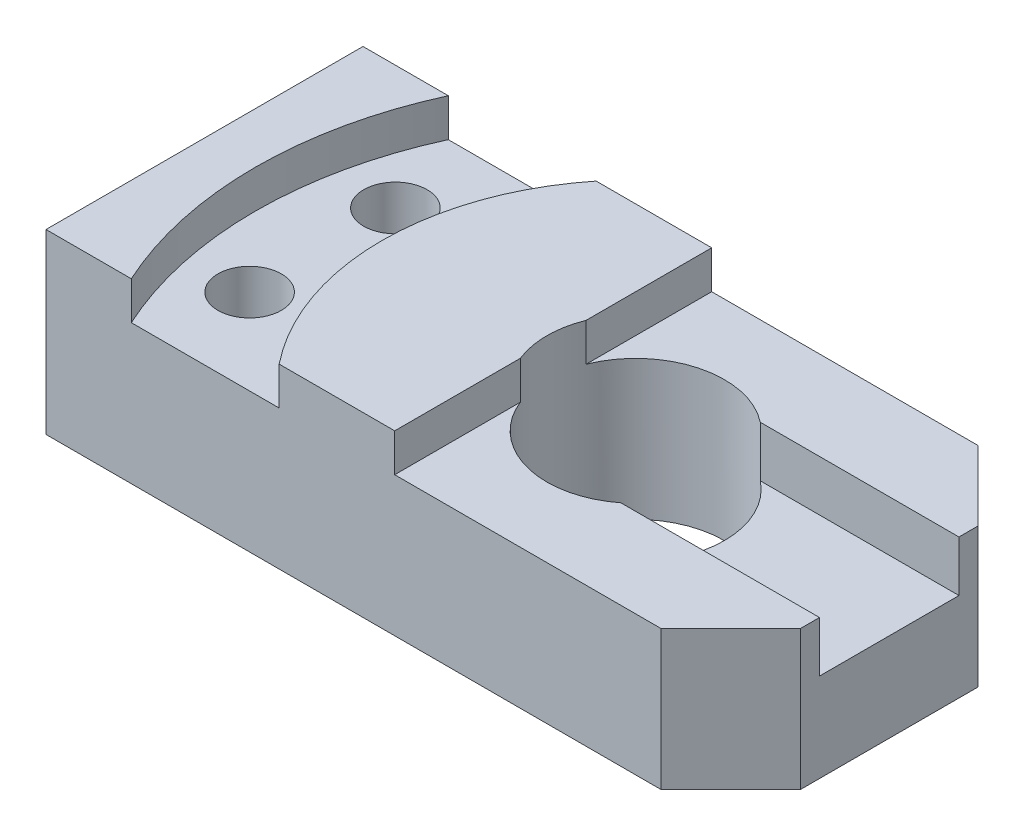
ISO-10303-21;
HEADER;
FILE_DESCRIPTION(('STEP AP214'),'2;1');
FILE_NAME('part.step','',(''),(''),'','','');
FILE_SCHEMA(('AUTOMOTIVE_DESIGN { 1 0 10303 214 1 1 1 1 }'));
ENDSEC;
DATA;
#1=APPLICATION_CONTEXT('core data for automotive mechanical design processes');
#2=APPLICATION_PROTOCOL_DEFINITION('international standard','automotive_design',2000,#1);
#3=PRODUCT_CONTEXT('',#1,'mechanical');
#4=PRODUCT('Part','Part','',(#3));
#5=PRODUCT_RELATED_PRODUCT_CATEGORY('part','',(#4));
#6=PRODUCT_DEFINITION_FORMATION('','',#4);
#7=PRODUCT_DEFINITION_CONTEXT('part definition',#1,'design');
#8=PRODUCT_DEFINITION('design','',#6,#7);
#9=PRODUCT_DEFINITION_SHAPE('','',#8);
#10=(LENGTH_UNIT() NAMED_UNIT(*) SI_UNIT(.MILLI.,.METRE.));
#11=(NAMED_UNIT(*) PLANE_ANGLE_UNIT() SI_UNIT($,.RADIAN.));
#12=(NAMED_UNIT(*) SI_UNIT($,.STERADIAN.) SOLID_ANGLE_UNIT());
#13=UNCERTAINTY_MEASURE_WITH_UNIT(LENGTH_MEASURE(1.E-05),#10,'distance_accuracy_value','');
#14=(GEOMETRIC_REPRESENTATION_CONTEXT(3) GLOBAL_UNCERTAINTY_ASSIGNED_CONTEXT((#13)) GLOBAL_UNIT_ASSIGNED_CONTEXT((#10,
#11,#12)) REPRESENTATION_CONTEXT('',''));
#15=CARTESIAN_POINT('',(0.,0.,0.));
#16=DIRECTION('',(0.,0.,1.));
#17=DIRECTION('',(1.,0.,0.));
#18=AXIS2_PLACEMENT_3D('',#15,#16,#17);
#19=CARTESIAN_POINT('',(0.,28.,0.));
#20=DIRECTION('',(0.,1.,0.));
#21=DIRECTION('',(0.,0.,1.));
#22=AXIS2_PLACEMENT_3D('',#19,#20,#21);
#23=PLANE('',#22);
#24=CARTESIAN_POINT('',(14.,28.,0.));
#25=DIRECTION('',(0.,-1.,0.));
#26=DIRECTION('',(0.,0.,1.));
#27=AXIS2_PLACEMENT_3D('',#24,#25,#26);
#28=CIRCLE('',#27,40.);
#29=CARTESIAN_POINT('',(-17.224989991992,28.,25.));
#30=VERTEX_POINT('',#29);
#31=CARTESIAN_POINT('',(-17.224989991992,28.,-25.));
#32=VERTEX_POINT('',#31);
#33=EDGE_CURVE('E176',#30,#32,#28,.T.);
#34=ORIENTED_EDGE('',*,*,#33,.F.);
#35=DIRECTION('',(1.,0.,0.));
#36=VECTOR('',#35,1.);
#37=CARTESIAN_POINT('',(-54.,28.,25.));
#38=LINE('',#37,#36);
#39=CARTESIAN_POINT('',(1.,28.,25.));
#40=VERTEX_POINT('',#39);
#41=EDGE_CURVE('E257',#30,#40,#38,.T.);
#42=ORIENTED_EDGE('',*,*,#41,.T.);
#43=DIRECTION('',(0.,0.,1.));
#44=VECTOR('',#43,1.);
#45=CARTESIAN_POINT('',(1.,28.,11.));
#46=LINE('',#45,#44);
#47=CARTESIAN_POINT('',(1.,28.,5.19615242270664));
#48=VERTEX_POINT('',#47);
#49=EDGE_CURVE('E231',#48,#40,#46,.T.);
#50=ORIENTED_EDGE('',*,*,#49,.F.);
#51=CARTESIAN_POINT('',(14.,28.,0.));
#52=DIRECTION('',(0.,1.,0.));
#53=DIRECTION('',(0.,0.,1.));
#54=AXIS2_PLACEMENT_3D('',#51,#52,#53);
#55=CIRCLE('',#54,14.);
#56=CARTESIAN_POINT('',(1.,28.,-5.19615242270664));
#57=VERTEX_POINT('',#56);
#58=EDGE_CURVE('E239',#57,#48,#55,.T.);
#59=ORIENTED_EDGE('',*,*,#58,.F.);
#60=CARTESIAN_POINT('',(1.,28.,-25.));
#61=VERTEX_POINT('',#60);
#62=EDGE_CURVE('E234',#61,#57,#46,.T.);
#63=ORIENTED_EDGE('',*,*,#62,.F.);
#64=DIRECTION('',(-1.,0.,0.));
#65=VECTOR('',#64,1.);
#66=CARTESIAN_POINT('',(54.,28.,-25.));
#67=LINE('',#66,#65);
#68=EDGE_CURVE('E252',#61,#32,#67,.T.);
#69=ORIENTED_EDGE('',*,*,#68,.T.);
#70=EDGE_LOOP('',(#34,#42,#50,#59,#63,#69));
#71=FACE_BOUND('',#70,.T.);
#72=ADVANCED_FACE('F43',(#71),#23,.T.);
#73=CARTESIAN_POINT('',(14.,22.,11.));
#74=DIRECTION('',(0.,-1.,0.));
#75=DIRECTION('',(0.,0.,-1.));
#76=AXIS2_PLACEMENT_3D('',#73,#74,#75);
#77=PLANE('',#76);
#78=DIRECTION('',(1.,0.,0.));
#79=VECTOR('',#78,1.);
#80=CARTESIAN_POINT('',(1.,22.,25.));
#81=LINE('',#80,#79);
#82=CARTESIAN_POINT('',(1.,22.,25.));
#83=VERTEX_POINT('',#82);
#84=CARTESIAN_POINT('',(43.,22.,25.));
#85=VERTEX_POINT('',#84);
#86=EDGE_CURVE('E236',#83,#85,#81,.T.);
#87=ORIENTED_EDGE('',*,*,#86,.T.);
#88=DIRECTION('',(-0.707106781186548,0.,0.707106781186547));
#89=VECTOR('',#88,1.);
#90=CARTESIAN_POINT('',(54.,22.,14.));
#91=LINE('',#90,#89);
#92=CARTESIAN_POINT('',(54.,22.,14.));
#93=VERTEX_POINT('',#92);
#94=EDGE_CURVE('E11',#85,#93,#91,.F.);
#95=ORIENTED_EDGE('',*,*,#94,.T.);
#96=DIRECTION('',(0.,0.,-1.));
#97=VECTOR('',#96,1.);
#98=CARTESIAN_POINT('',(54.,22.,11.));
#99=LINE('',#98,#97);
#100=CARTESIAN_POINT('',(54.,22.,11.));
#101=VERTEX_POINT('',#100);
#102=EDGE_CURVE('E247',#93,#101,#99,.T.);
#103=ORIENTED_EDGE('',*,*,#102,.T.);
#104=DIRECTION('',(1.,0.,0.));
#105=VECTOR('',#104,1.);
#106=CARTESIAN_POINT('',(14.,22.,11.));
#107=LINE('',#106,#105);
#108=CARTESIAN_POINT('',(22.6602540378444,22.,11.));
#109=VERTEX_POINT('',#108);
#110=EDGE_CURVE('E213',#109,#101,#107,.T.);
#111=ORIENTED_EDGE('',*,*,#110,.F.);
#112=CARTESIAN_POINT('',(14.,22.,0.));
#113=DIRECTION('',(0.,-1.,0.));
#114=DIRECTION('',(0.,0.,-1.));
#115=AXIS2_PLACEMENT_3D('',#112,#113,#114);
#116=CIRCLE('',#115,14.);
#117=CARTESIAN_POINT('',(1.,22.,5.19615242270664));
#118=VERTEX_POINT('',#117);
#119=EDGE_CURVE('E273',#109,#118,#116,.T.);
#120=ORIENTED_EDGE('',*,*,#119,.T.);
#121=DIRECTION('',(0.,0.,-1.));
#122=VECTOR('',#121,1.);
#123=CARTESIAN_POINT('',(1.,22.,25.));
#124=LINE('',#123,#122);
#125=EDGE_CURVE('E226',#83,#118,#124,.T.);
#126=ORIENTED_EDGE('',*,*,#125,.F.);
#127=EDGE_LOOP('',(#87,#95,#103,#111,#120,#126));
#128=FACE_BOUND('',#127,.T.);
#129=ADVANCED_FACE('F336',(#128),#77,.F.);
#130=CARTESIAN_POINT('',(14.,28.,0.));
#131=DIRECTION('',(0.,1.,0.));
#132=DIRECTION('',(0.,0.,1.));
#133=AXIS2_PLACEMENT_3D('',#130,#131,#132);
#134=CIRCLE('',#133,60.);
#135=CARTESIAN_POINT('',(-40.5435605731786,28.,-25.));
#136=VERTEX_POINT('',#135);
#137=CARTESIAN_POINT('',(-40.5435605731786,28.,25.));
#138=VERTEX_POINT('',#137);
#139=EDGE_CURVE('E186',#136,#138,#134,.T.);
#140=ORIENTED_EDGE('',*,*,#139,.F.);
#141=CARTESIAN_POINT('',(-54.,28.,-25.));
#142=VERTEX_POINT('',#141);
#143=EDGE_CURVE('E251',#136,#142,#67,.T.);
#144=ORIENTED_EDGE('',*,*,#143,.T.);
#145=DIRECTION('',(0.,0.,1.));
#146=VECTOR('',#145,1.);
#147=CARTESIAN_POINT('',(-54.,28.,-25.));
#148=LINE('',#147,#146);
#149=CARTESIAN_POINT('',(-54.,28.,25.));
#150=VERTEX_POINT('',#149);
#151=EDGE_CURVE('E254',#142,#150,#148,.T.);
#152=ORIENTED_EDGE('',*,*,#151,.T.);
#153=EDGE_CURVE('E260',#150,#138,#38,.T.);
#154=ORIENTED_EDGE('',*,*,#153,.T.);
#155=EDGE_LOOP('',(#140,#144,#152,#154));
#156=FACE_BOUND('',#155,.T.);
#157=ADVANCED_FACE('F342',(#156),#23,.T.);
#158=CARTESIAN_POINT('',(54.,28.,25.));
#159=DIRECTION('',(-1.,0.,0.));
#160=DIRECTION('',(0.,0.,1.));
#161=AXIS2_PLACEMENT_3D('',#158,#159,#160);
#162=PLANE('',#161);
#163=DIRECTION('',(0.,0.,-1.));
#164=VECTOR('',#163,1.);
#165=CARTESIAN_POINT('',(54.,0.,25.));
#166=LINE('',#165,#164);
#167=CARTESIAN_POINT('',(54.,0.,14.));
#168=VERTEX_POINT('',#167);
#169=CARTESIAN_POINT('',(54.,0.,-14.));
#170=VERTEX_POINT('',#169);
#171=EDGE_CURVE('E249',#168,#170,#166,.T.);
#172=ORIENTED_EDGE('',*,*,#171,.T.);
#173=DIRECTION('',(0.,1.,0.));
#174=VECTOR('',#173,1.);
#175=CARTESIAN_POINT('',(54.,28.,-14.));
#176=LINE('',#175,#174);
#177=CARTESIAN_POINT('',(54.,22.,-14.));
#178=VERTEX_POINT('',#177);
#179=EDGE_CURVE('E303',#170,#178,#176,.T.);
#180=ORIENTED_EDGE('',*,*,#179,.T.);
#181=CARTESIAN_POINT('',(54.,22.,-11.));
#182=VERTEX_POINT('',#181);
#183=EDGE_CURVE('E244',#182,#178,#99,.T.);
#184=ORIENTED_EDGE('',*,*,#183,.F.);
#185=DIRECTION('',(0.,1.,0.));
#186=VECTOR('',#185,1.);
#187=CARTESIAN_POINT('',(54.,22.,-11.));
#188=LINE('',#187,#186);
#189=CARTESIAN_POINT('',(54.,14.,-11.));
#190=VERTEX_POINT('',#189);
#191=EDGE_CURVE('E215',#190,#182,#188,.T.);
#192=ORIENTED_EDGE('',*,*,#191,.F.);
#193=DIRECTION('',(0.,0.,-1.));
#194=VECTOR('',#193,1.);
#195=CARTESIAN_POINT('',(54.,14.,11.));
#196=LINE('',#195,#194);
#197=CARTESIAN_POINT('',(54.,14.,11.));
#198=VERTEX_POINT('',#197);
#199=EDGE_CURVE('E209',#198,#190,#196,.T.);
#200=ORIENTED_EDGE('',*,*,#199,.F.);
#201=DIRECTION('',(0.,-1.,0.));
#202=VECTOR('',#201,1.);
#203=CARTESIAN_POINT('',(54.,22.,11.));
#204=LINE('',#203,#202);
#205=EDGE_CURVE('E204',#101,#198,#204,.T.);
#206=ORIENTED_EDGE('',*,*,#205,.F.);
#207=ORIENTED_EDGE('',*,*,#102,.F.);
#208=DIRECTION('',(0.,-1.,0.));
#209=VECTOR('',#208,1.);
#210=CARTESIAN_POINT('',(54.,28.,14.));
#211=LINE('',#210,#209);
#212=EDGE_CURVE('E297',#93,#168,#211,.T.);
#213=ORIENTED_EDGE('',*,*,#212,.T.);
#214=EDGE_LOOP('',(#172,#180,#184,#192,#200,#206,#207,#213));
#215=FACE_BOUND('',#214,.T.);
#216=ADVANCED_FACE('F352',(#215),#162,.F.);
#217=CARTESIAN_POINT('',(-54.,28.,-25.));
#218=DIRECTION('',(0.,0.,1.));
#219=DIRECTION('',(1.,0.,0.));
#220=AXIS2_PLACEMENT_3D('',#217,#218,#219);
#221=PLANE('',#220);
#222=DIRECTION('',(-1.,0.,0.));
#223=VECTOR('',#222,1.);
#224=CARTESIAN_POINT('',(-17.224989991992,22.,-25.));
#225=LINE('',#224,#223);
#226=CARTESIAN_POINT('',(-17.224989991992,22.,-25.));
#227=VERTEX_POINT('',#226);
#228=CARTESIAN_POINT('',(-40.5435605731786,22.,-25.));
#229=VERTEX_POINT('',#228);
#230=EDGE_CURVE('E184',#227,#229,#225,.T.);
#231=ORIENTED_EDGE('',*,*,#230,.F.);
#232=DIRECTION('',(0.,1.,0.));
#233=VECTOR('',#232,1.);
#234=CARTESIAN_POINT('',(-17.224989991992,22.,-25.));
#235=LINE('',#234,#233);
#236=EDGE_CURVE('E171',#227,#32,#235,.T.);
#237=ORIENTED_EDGE('',*,*,#236,.T.);
#238=ORIENTED_EDGE('',*,*,#68,.F.);
#239=DIRECTION('',(0.,1.,0.));
#240=VECTOR('',#239,1.);
#241=CARTESIAN_POINT('',(1.,28.,-25.));
#242=LINE('',#241,#240);
#243=CARTESIAN_POINT('',(1.,22.,-25.));
#244=VERTEX_POINT('',#243);
#245=EDGE_CURVE('E233',#244,#61,#242,.T.);
#246=ORIENTED_EDGE('',*,*,#245,.F.);
#247=DIRECTION('',(1.,0.,0.));
#248=VECTOR('',#247,1.);
#249=CARTESIAN_POINT('',(1.,22.,-25.));
#250=LINE('',#249,#248);
#251=CARTESIAN_POINT('',(43.,22.,-25.));
#252=VERTEX_POINT('',#251);
#253=EDGE_CURVE('E240',#244,#252,#250,.T.);
#254=ORIENTED_EDGE('',*,*,#253,.T.);
#255=DIRECTION('',(0.,-1.,0.));
#256=VECTOR('',#255,1.);
#257=CARTESIAN_POINT('',(43.,28.,-25.));
#258=LINE('',#257,#256);
#259=CARTESIAN_POINT('',(43.,0.,-25.));
#260=VERTEX_POINT('',#259);
#261=EDGE_CURVE('E291',#252,#260,#258,.T.);
#262=ORIENTED_EDGE('',*,*,#261,.T.);
#263=DIRECTION('',(-1.,0.,0.));
#264=VECTOR('',#263,1.);
#265=CARTESIAN_POINT('',(-54.,0.,-25.));
#266=LINE('',#265,#264);
#267=CARTESIAN_POINT('',(-54.,0.,-25.));
#268=VERTEX_POINT('',#267);
#269=EDGE_CURVE('E261',#260,#268,#266,.T.);
#270=ORIENTED_EDGE('',*,*,#269,.T.);
#271=DIRECTION('',(0.,-1.,0.));
#272=VECTOR('',#271,1.);
#273=CARTESIAN_POINT('',(-54.,28.,-25.));
#274=LINE('',#273,#272);
#275=EDGE_CURVE('E275',#142,#268,#274,.T.);
#276=ORIENTED_EDGE('',*,*,#275,.F.);
#277=ORIENTED_EDGE('',*,*,#143,.F.);
#278=DIRECTION('',(0.,1.,0.));
#279=VECTOR('',#278,1.);
#280=CARTESIAN_POINT('',(-40.5435605731786,22.,-25.));
#281=LINE('',#280,#279);
#282=EDGE_CURVE('E181',#229,#136,#281,.T.);
#283=ORIENTED_EDGE('',*,*,#282,.F.);
#284=EDGE_LOOP('',(#231,#237,#238,#246,#254,#262,#270,#276,#277,#283));
#285=FACE_BOUND('',#284,.T.);
#286=ADVANCED_FACE('F192',(#285),#221,.F.);
#287=CARTESIAN_POINT('',(-54.,28.,-25.));
#288=DIRECTION('',(1.,0.,0.));
#289=DIRECTION('',(0.,0.,-1.));
#290=AXIS2_PLACEMENT_3D('',#287,#288,#289);
#291=PLANE('',#290);
#292=DIRECTION('',(0.,0.,1.));
#293=VECTOR('',#292,1.);
#294=CARTESIAN_POINT('',(-54.,0.,-25.));
#295=LINE('',#294,#293);
#296=CARTESIAN_POINT('',(-54.,0.,25.));
#297=VERTEX_POINT('',#296);
#298=EDGE_CURVE('E264',#268,#297,#295,.T.);
#299=ORIENTED_EDGE('',*,*,#298,.T.);
#300=DIRECTION('',(0.,-1.,0.));
#301=VECTOR('',#300,1.);
#302=CARTESIAN_POINT('',(-54.,28.,25.));
#303=LINE('',#302,#301);
#304=EDGE_CURVE('E258',#150,#297,#303,.T.);
#305=ORIENTED_EDGE('',*,*,#304,.F.);
#306=ORIENTED_EDGE('',*,*,#151,.F.);
#307=ORIENTED_EDGE('',*,*,#275,.T.);
#308=EDGE_LOOP('',(#299,#305,#306,#307));
#309=FACE_BOUND('',#308,.T.);
#310=ADVANCED_FACE('F368',(#309),#291,.F.);
#311=CARTESIAN_POINT('',(43.,28.,25.));
#312=DIRECTION('',(0.,0.,-1.));
#313=DIRECTION('',(-1.,0.,0.));
#314=AXIS2_PLACEMENT_3D('',#311,#312,#313);
#315=PLANE('',#314);
#316=ORIENTED_EDGE('',*,*,#41,.F.);
#317=DIRECTION('',(0.,1.,0.));
#318=VECTOR('',#317,1.);
#319=CARTESIAN_POINT('',(-17.224989991992,22.,25.));
#320=LINE('',#319,#318);
#321=CARTESIAN_POINT('',(-17.224989991992,22.,25.));
#322=VERTEX_POINT('',#321);
#323=EDGE_CURVE('E199',#322,#30,#320,.T.);
#324=ORIENTED_EDGE('',*,*,#323,.F.);
#325=DIRECTION('',(1.,0.,0.));
#326=VECTOR('',#325,1.);
#327=CARTESIAN_POINT('',(-40.5435605731786,22.,25.));
#328=LINE('',#327,#326);
#329=CARTESIAN_POINT('',(-40.5435605731786,22.,25.));
#330=VERTEX_POINT('',#329);
#331=EDGE_CURVE('E185',#330,#322,#328,.T.);
#332=ORIENTED_EDGE('',*,*,#331,.F.);
#333=DIRECTION('',(0.,1.,0.));
#334=VECTOR('',#333,1.);
#335=CARTESIAN_POINT('',(-40.5435605731786,22.,25.));
#336=LINE('',#335,#334);
#337=EDGE_CURVE('E205',#330,#138,#336,.T.);
#338=ORIENTED_EDGE('',*,*,#337,.T.);
#339=ORIENTED_EDGE('',*,*,#153,.F.);
#340=ORIENTED_EDGE('',*,*,#304,.T.);
#341=DIRECTION('',(1.,0.,0.));
#342=VECTOR('',#341,1.);
#343=CARTESIAN_POINT('',(43.,0.,25.));
#344=LINE('',#343,#342);
#345=CARTESIAN_POINT('',(43.,0.,25.));
#346=VERTEX_POINT('',#345);
#347=EDGE_CURVE('E270',#297,#346,#344,.T.);
#348=ORIENTED_EDGE('',*,*,#347,.T.);
#349=DIRECTION('',(0.,1.,0.));
#350=VECTOR('',#349,1.);
#351=CARTESIAN_POINT('',(43.,28.,25.));
#352=LINE('',#351,#350);
#353=EDGE_CURVE('E52',#346,#85,#352,.T.);
#354=ORIENTED_EDGE('',*,*,#353,.T.);
#355=ORIENTED_EDGE('',*,*,#86,.F.);
#356=DIRECTION('',(0.,-1.,0.));
#357=VECTOR('',#356,1.);
#358=CARTESIAN_POINT('',(1.,28.,25.));
#359=LINE('',#358,#357);
#360=EDGE_CURVE('E216',#40,#83,#359,.T.);
#361=ORIENTED_EDGE('',*,*,#360,.F.);
#362=EDGE_LOOP('',(#316,#324,#332,#338,#339,#340,#348,#354,#355,#361));
#363=FACE_BOUND('',#362,.T.);
#364=ADVANCED_FACE('F369',(#363),#315,.F.);
#365=CARTESIAN_POINT('',(0.,0.,0.));
#366=DIRECTION('',(0.,1.,0.));
#367=DIRECTION('',(0.,0.,1.));
#368=AXIS2_PLACEMENT_3D('',#365,#366,#367);
#369=PLANE('',#368);
#370=CARTESIAN_POINT('',(-35.3853627580158,0.,-11.4974013184257));
#371=DIRECTION('',(0.,1.,0.));
#372=DIRECTION('',(0.,0.,1.));
#373=AXIS2_PLACEMENT_3D('',#370,#371,#372);
#374=CIRCLE('',#373,5.);
#375=CARTESIAN_POINT('',(-35.3853627580158,0.,-6.49740131842571));
#376=VERTEX_POINT('',#375);
#377=EDGE_CURVE('E307',#376,#376,#374,.T.);
#378=ORIENTED_EDGE('',*,*,#377,.T.);
#379=EDGE_LOOP('',(#378));
#380=FACE_BOUND('',#379,.T.);
#381=CARTESIAN_POINT('',(-35.3853627580158,0.,11.4974013184257));
#382=DIRECTION('',(0.,1.,0.));
#383=DIRECTION('',(0.,0.,1.));
#384=AXIS2_PLACEMENT_3D('',#381,#382,#383);
#385=CIRCLE('',#384,5.);
#386=CARTESIAN_POINT('',(-35.3853627580158,0.,16.4974013184257));
#387=VERTEX_POINT('',#386);
#388=EDGE_CURVE('E313',#387,#387,#385,.T.);
#389=ORIENTED_EDGE('',*,*,#388,.T.);
#390=EDGE_LOOP('',(#389));
#391=FACE_BOUND('',#390,.T.);
#392=CARTESIAN_POINT('',(14.,0.,0.));
#393=DIRECTION('',(0.,1.,0.));
#394=DIRECTION('',(0.,0.,1.));
#395=AXIS2_PLACEMENT_3D('',#392,#393,#394);
#396=CIRCLE('',#395,14.);
#397=CARTESIAN_POINT('',(14.,0.,14.));
#398=VERTEX_POINT('',#397);
#399=EDGE_CURVE('E245',#398,#398,#396,.T.);
#400=ORIENTED_EDGE('',*,*,#399,.T.);
#401=EDGE_LOOP('',(#400));
#402=FACE_BOUND('',#401,.T.);
#403=ORIENTED_EDGE('',*,*,#269,.F.);
#404=DIRECTION('',(-0.707106781186546,0.,-0.707106781186549));
#405=VECTOR('',#404,1.);
#406=CARTESIAN_POINT('',(43.,0.,-25.));
#407=LINE('',#406,#405);
#408=EDGE_CURVE('E296',#260,#170,#407,.F.);
#409=ORIENTED_EDGE('',*,*,#408,.T.);
#410=ORIENTED_EDGE('',*,*,#171,.F.);
#411=DIRECTION('',(0.707106781186548,0.,-0.707106781186547));
#412=VECTOR('',#411,1.);
#413=CARTESIAN_POINT('',(54.,0.,14.));
#414=LINE('',#413,#412);
#415=EDGE_CURVE('E298',#168,#346,#414,.F.);
#416=ORIENTED_EDGE('',*,*,#415,.T.);
#417=ORIENTED_EDGE('',*,*,#347,.F.);
#418=ORIENTED_EDGE('',*,*,#298,.F.);
#419=EDGE_LOOP('',(#403,#409,#410,#416,#417,#418));
#420=FACE_BOUND('',#419,.T.);
#421=ADVANCED_FACE('F322',(#380,#391,#402,#420),#369,.F.);
#422=ORIENTED_EDGE('',*,*,#183,.T.);
#423=DIRECTION('',(0.707106781186546,0.,0.707106781186549));
#424=VECTOR('',#423,1.);
#425=CARTESIAN_POINT('',(43.,22.,-25.));
#426=LINE('',#425,#424);
#427=EDGE_CURVE('E304',#178,#252,#426,.F.);
#428=ORIENTED_EDGE('',*,*,#427,.T.);
#429=ORIENTED_EDGE('',*,*,#253,.F.);
#430=CARTESIAN_POINT('',(1.,22.,-5.19615242270664));
#431=VERTEX_POINT('',#430);
#432=EDGE_CURVE('E227',#431,#244,#124,.T.);
#433=ORIENTED_EDGE('',*,*,#432,.F.);
#434=CARTESIAN_POINT('',(22.6602540378444,22.,-11.));
#435=VERTEX_POINT('',#434);
#436=EDGE_CURVE('E277',#431,#435,#116,.T.);
#437=ORIENTED_EDGE('',*,*,#436,.T.);
#438=DIRECTION('',(1.,0.,0.));
#439=VECTOR('',#438,1.);
#440=CARTESIAN_POINT('',(14.,22.,-11.));
#441=LINE('',#440,#439);
#442=EDGE_CURVE('E217',#435,#182,#441,.T.);
#443=ORIENTED_EDGE('',*,*,#442,.T.);
#444=EDGE_LOOP('',(#422,#428,#429,#433,#437,#443));
#445=FACE_BOUND('',#444,.T.);
#446=ADVANCED_FACE('F347',(#445),#77,.F.);
#447=CARTESIAN_POINT('',(14.,0.,0.));
#448=DIRECTION('',(0.,1.,0.));
#449=DIRECTION('',(0.,0.,1.));
#450=AXIS2_PLACEMENT_3D('',#447,#448,#449);
#451=CYLINDRICAL_SURFACE('',#450,14.);
#452=ORIENTED_EDGE('',*,*,#119,.F.);
#453=DIRECTION('',(0.,1.,0.));
#454=VECTOR('',#453,1.);
#455=CARTESIAN_POINT('',(22.6602540378444,0.,11.));
#456=LINE('',#455,#454);
#457=CARTESIAN_POINT('',(22.6602540378444,14.,11.));
#458=VERTEX_POINT('',#457);
#459=EDGE_CURVE('E288',#109,#458,#456,.F.);
#460=ORIENTED_EDGE('',*,*,#459,.T.);
#461=CARTESIAN_POINT('',(14.,14.,0.));
#462=DIRECTION('',(0.,-1.,0.));
#463=DIRECTION('',(0.,0.,-1.));
#464=AXIS2_PLACEMENT_3D('',#461,#462,#463);
#465=CIRCLE('',#464,14.);
#466=CARTESIAN_POINT('',(22.6602540378444,14.,-11.));
#467=VERTEX_POINT('',#466);
#468=EDGE_CURVE('E282',#458,#467,#465,.F.);
#469=ORIENTED_EDGE('',*,*,#468,.T.);
#470=DIRECTION('',(0.,1.,0.));
#471=VECTOR('',#470,1.);
#472=CARTESIAN_POINT('',(22.6602540378444,0.,-11.));
#473=LINE('',#472,#471);
#474=EDGE_CURVE('E289',#467,#435,#473,.T.);
#475=ORIENTED_EDGE('',*,*,#474,.T.);
#476=ORIENTED_EDGE('',*,*,#436,.F.);
#477=DIRECTION('',(0.,1.,0.));
#478=VECTOR('',#477,1.);
#479=CARTESIAN_POINT('',(1.,0.,-5.19615242270664));
#480=LINE('',#479,#478);
#481=EDGE_CURVE('E283',#57,#431,#480,.F.);
#482=ORIENTED_EDGE('',*,*,#481,.F.);
#483=ORIENTED_EDGE('',*,*,#58,.T.);
#484=DIRECTION('',(0.,1.,0.));
#485=VECTOR('',#484,1.);
#486=CARTESIAN_POINT('',(1.,0.,5.19615242270664));
#487=LINE('',#486,#485);
#488=EDGE_CURVE('E276',#118,#48,#487,.T.);
#489=ORIENTED_EDGE('',*,*,#488,.F.);
#490=EDGE_LOOP('',(#452,#460,#469,#475,#476,#482,#483,#489));
#491=FACE_BOUND('',#490,.T.);
#492=ORIENTED_EDGE('',*,*,#399,.F.);
#493=EDGE_LOOP('',(#492));
#494=FACE_BOUND('',#493,.T.);
#495=ADVANCED_FACE('F399',(#491,#494),#451,.F.);
#496=CARTESIAN_POINT('',(1.,0.,0.));
#497=DIRECTION('',(1.,0.,0.));
#498=DIRECTION('',(0.,0.,-1.));
#499=AXIS2_PLACEMENT_3D('',#496,#497,#498);
#500=PLANE('',#499);
#501=ORIENTED_EDGE('',*,*,#488,.T.);
#502=ORIENTED_EDGE('',*,*,#49,.T.);
#503=ORIENTED_EDGE('',*,*,#360,.T.);
#504=ORIENTED_EDGE('',*,*,#125,.T.);
#505=EDGE_LOOP('',(#501,#502,#503,#504));
#506=FACE_BOUND('',#505,.T.);
#507=ADVANCED_FACE('F394',(#506),#500,.T.);
#508=ORIENTED_EDGE('',*,*,#481,.T.);
#509=ORIENTED_EDGE('',*,*,#432,.T.);
#510=ORIENTED_EDGE('',*,*,#245,.T.);
#511=ORIENTED_EDGE('',*,*,#62,.T.);
#512=EDGE_LOOP('',(#508,#509,#510,#511));
#513=FACE_BOUND('',#512,.T.);
#514=ADVANCED_FACE('F393',(#513),#500,.T.);
#515=CARTESIAN_POINT('',(14.,22.,11.));
#516=DIRECTION('',(0.,0.,1.));
#517=DIRECTION('',(0.,-1.,0.));
#518=AXIS2_PLACEMENT_3D('',#515,#516,#517);
#519=PLANE('',#518);
#520=ORIENTED_EDGE('',*,*,#110,.T.);
#521=ORIENTED_EDGE('',*,*,#205,.T.);
#522=DIRECTION('',(1.,0.,0.));
#523=VECTOR('',#522,1.);
#524=CARTESIAN_POINT('',(14.,14.,11.));
#525=LINE('',#524,#523);
#526=EDGE_CURVE('E211',#458,#198,#525,.T.);
#527=ORIENTED_EDGE('',*,*,#526,.F.);
#528=ORIENTED_EDGE('',*,*,#459,.F.);
#529=EDGE_LOOP('',(#520,#521,#527,#528));
#530=FACE_BOUND('',#529,.T.);
#531=ADVANCED_FACE('F384',(#530),#519,.F.);
#532=CARTESIAN_POINT('',(14.,22.,-11.));
#533=DIRECTION('',(0.,0.,-1.));
#534=DIRECTION('',(0.,1.,0.));
#535=AXIS2_PLACEMENT_3D('',#532,#533,#534);
#536=PLANE('',#535);
#537=DIRECTION('',(1.,0.,0.));
#538=VECTOR('',#537,1.);
#539=CARTESIAN_POINT('',(14.,14.,-11.));
#540=LINE('',#539,#538);
#541=EDGE_CURVE('E224',#467,#190,#540,.T.);
#542=ORIENTED_EDGE('',*,*,#541,.T.);
#543=ORIENTED_EDGE('',*,*,#191,.T.);
#544=ORIENTED_EDGE('',*,*,#442,.F.);
#545=ORIENTED_EDGE('',*,*,#474,.F.);
#546=EDGE_LOOP('',(#542,#543,#544,#545));
#547=FACE_BOUND('',#546,.T.);
#548=ADVANCED_FACE('F378',(#547),#536,.F.);
#549=CARTESIAN_POINT('',(14.,14.,11.));
#550=DIRECTION('',(0.,-1.,0.));
#551=DIRECTION('',(0.,0.,-1.));
#552=AXIS2_PLACEMENT_3D('',#549,#550,#551);
#553=PLANE('',#552);
#554=ORIENTED_EDGE('',*,*,#526,.T.);
#555=ORIENTED_EDGE('',*,*,#199,.T.);
#556=ORIENTED_EDGE('',*,*,#541,.F.);
#557=ORIENTED_EDGE('',*,*,#468,.F.);
#558=EDGE_LOOP('',(#554,#555,#556,#557));
#559=FACE_BOUND('',#558,.T.);
#560=ADVANCED_FACE('F385',(#559),#553,.F.);
#561=CARTESIAN_POINT('',(43.,28.,-25.));
#562=DIRECTION('',(-0.707106781186549,0.,0.707106781186546));
#563=DIRECTION('',(0.,-1.,0.));
#564=AXIS2_PLACEMENT_3D('',#561,#562,#563);
#565=PLANE('',#564);
#566=ORIENTED_EDGE('',*,*,#427,.F.);
#567=ORIENTED_EDGE('',*,*,#179,.F.);
#568=ORIENTED_EDGE('',*,*,#408,.F.);
#569=ORIENTED_EDGE('',*,*,#261,.F.);
#570=EDGE_LOOP('',(#566,#567,#568,#569));
#571=FACE_BOUND('',#570,.T.);
#572=ADVANCED_FACE('F390',(#571),#565,.F.);
#573=CARTESIAN_POINT('',(54.,28.,14.));
#574=DIRECTION('',(-0.707106781186547,0.,-0.707106781186548));
#575=DIRECTION('',(0.,-1.,0.));
#576=AXIS2_PLACEMENT_3D('',#573,#574,#575);
#577=PLANE('',#576);
#578=ORIENTED_EDGE('',*,*,#94,.F.);
#579=ORIENTED_EDGE('',*,*,#353,.F.);
#580=ORIENTED_EDGE('',*,*,#415,.F.);
#581=ORIENTED_EDGE('',*,*,#212,.F.);
#582=EDGE_LOOP('',(#578,#579,#580,#581));
#583=FACE_BOUND('',#582,.T.);
#584=ADVANCED_FACE('F46',(#583),#577,.F.);
#585=CARTESIAN_POINT('',(14.,22.,0.));
#586=DIRECTION('',(0.,1.,0.));
#587=DIRECTION('',(0.,0.,1.));
#588=AXIS2_PLACEMENT_3D('',#585,#586,#587);
#589=CYLINDRICAL_SURFACE('',#588,40.);
#590=ORIENTED_EDGE('',*,*,#33,.T.);
#591=ORIENTED_EDGE('',*,*,#236,.F.);
#592=CARTESIAN_POINT('',(14.,22.,0.));
#593=DIRECTION('',(0.,-1.,0.));
#594=DIRECTION('',(0.,0.,1.));
#595=AXIS2_PLACEMENT_3D('',#592,#593,#594);
#596=CIRCLE('',#595,40.);
#597=EDGE_CURVE('E172',#322,#227,#596,.T.);
#598=ORIENTED_EDGE('',*,*,#597,.F.);
#599=ORIENTED_EDGE('',*,*,#323,.T.);
#600=EDGE_LOOP('',(#590,#591,#598,#599));
#601=FACE_BOUND('',#600,.T.);
#602=ADVANCED_FACE('F173',(#601),#589,.T.);
#603=CARTESIAN_POINT('',(14.,22.,0.));
#604=DIRECTION('',(0.,1.,0.));
#605=DIRECTION('',(0.,0.,1.));
#606=AXIS2_PLACEMENT_3D('',#603,#604,#605);
#607=CYLINDRICAL_SURFACE('',#606,60.);
#608=ORIENTED_EDGE('',*,*,#139,.T.);
#609=ORIENTED_EDGE('',*,*,#337,.F.);
#610=CARTESIAN_POINT('',(14.,22.,0.));
#611=DIRECTION('',(0.,1.,0.));
#612=DIRECTION('',(0.,0.,1.));
#613=AXIS2_PLACEMENT_3D('',#610,#611,#612);
#614=CIRCLE('',#613,60.);
#615=EDGE_CURVE('E62',#229,#330,#614,.T.);
#616=ORIENTED_EDGE('',*,*,#615,.F.);
#617=ORIENTED_EDGE('',*,*,#282,.T.);
#618=EDGE_LOOP('',(#608,#609,#616,#617));
#619=FACE_BOUND('',#618,.T.);
#620=ADVANCED_FACE('F331',(#619),#607,.F.);
#621=CARTESIAN_POINT('',(14.,22.,0.));
#622=DIRECTION('',(0.,1.,0.));
#623=DIRECTION('',(0.,0.,1.));
#624=AXIS2_PLACEMENT_3D('',#621,#622,#623);
#625=PLANE('',#624);
#626=CARTESIAN_POINT('',(-35.3853627580158,22.,-11.4974013184257));
#627=DIRECTION('',(0.,1.,0.));
#628=DIRECTION('',(0.,0.,1.));
#629=AXIS2_PLACEMENT_3D('',#626,#627,#628);
#630=CIRCLE('',#629,5.);
#631=CARTESIAN_POINT('',(-35.3853627580158,22.,-6.49740131842571));
#632=VERTEX_POINT('',#631);
#633=EDGE_CURVE('E48',#632,#632,#630,.T.);
#634=ORIENTED_EDGE('',*,*,#633,.F.);
#635=EDGE_LOOP('',(#634));
#636=FACE_BOUND('',#635,.T.);
#637=CARTESIAN_POINT('',(-35.3853627580158,22.,11.4974013184257));
#638=DIRECTION('',(0.,1.,0.));
#639=DIRECTION('',(0.,0.,1.));
#640=AXIS2_PLACEMENT_3D('',#637,#638,#639);
#641=CIRCLE('',#640,5.);
#642=CARTESIAN_POINT('',(-35.3853627580158,22.,16.4974013184257));
#643=VERTEX_POINT('',#642);
#644=EDGE_CURVE('E310',#643,#643,#641,.T.);
#645=ORIENTED_EDGE('',*,*,#644,.F.);
#646=EDGE_LOOP('',(#645));
#647=FACE_BOUND('',#646,.T.);
#648=ORIENTED_EDGE('',*,*,#597,.T.);
#649=ORIENTED_EDGE('',*,*,#230,.T.);
#650=ORIENTED_EDGE('',*,*,#615,.T.);
#651=ORIENTED_EDGE('',*,*,#331,.T.);
#652=EDGE_LOOP('',(#648,#649,#650,#651));
#653=FACE_BOUND('',#652,.T.);
#654=ADVANCED_FACE('F183',(#636,#647,#653),#625,.T.);
#655=CARTESIAN_POINT('',(-35.3853627580158,0.,11.4974013184257));
#656=DIRECTION('',(0.,1.,0.));
#657=DIRECTION('',(0.,0.,1.));
#658=AXIS2_PLACEMENT_3D('',#655,#656,#657);
#659=CYLINDRICAL_SURFACE('',#658,5.);
#660=ORIENTED_EDGE('',*,*,#644,.T.);
#661=EDGE_LOOP('',(#660));
#662=FACE_BOUND('',#661,.T.);
#663=ORIENTED_EDGE('',*,*,#388,.F.);
#664=EDGE_LOOP('',(#663));
#665=FACE_BOUND('',#664,.T.);
#666=ADVANCED_FACE('F321',(#662,#665),#659,.F.);
#667=CARTESIAN_POINT('',(-35.3853627580158,0.,-11.4974013184257));
#668=DIRECTION('',(0.,1.,0.));
#669=DIRECTION('',(0.,0.,1.));
#670=AXIS2_PLACEMENT_3D('',#667,#668,#669);
#671=CYLINDRICAL_SURFACE('',#670,5.);
#672=ORIENTED_EDGE('',*,*,#633,.T.);
#673=EDGE_LOOP('',(#672));
#674=FACE_BOUND('',#673,.T.);
#675=ORIENTED_EDGE('',*,*,#377,.F.);
#676=EDGE_LOOP('',(#675));
#677=FACE_BOUND('',#676,.T.);
#678=ADVANCED_FACE('F328',(#674,#677),#671,.F.);
#679=CLOSED_SHELL('',(#72,#129,#157,#216,#286,#310,#364,#421,#446,#495,#507,#514,#531,#548,#560,
#572,#584,#602,#620,#654,#666,#678));
#680=MANIFOLD_SOLID_BREP('B2',#679);
#681=ADVANCED_BREP_SHAPE_REPRESENTATION('',(#18,#680),#14);
#682=SHAPE_DEFINITION_REPRESENTATION(#9,#681);
ENDSEC;
END-ISO-10303-21;
